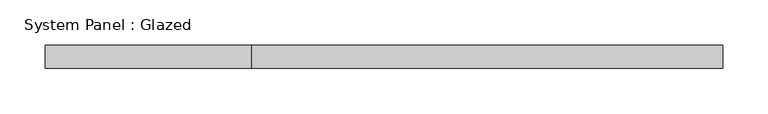
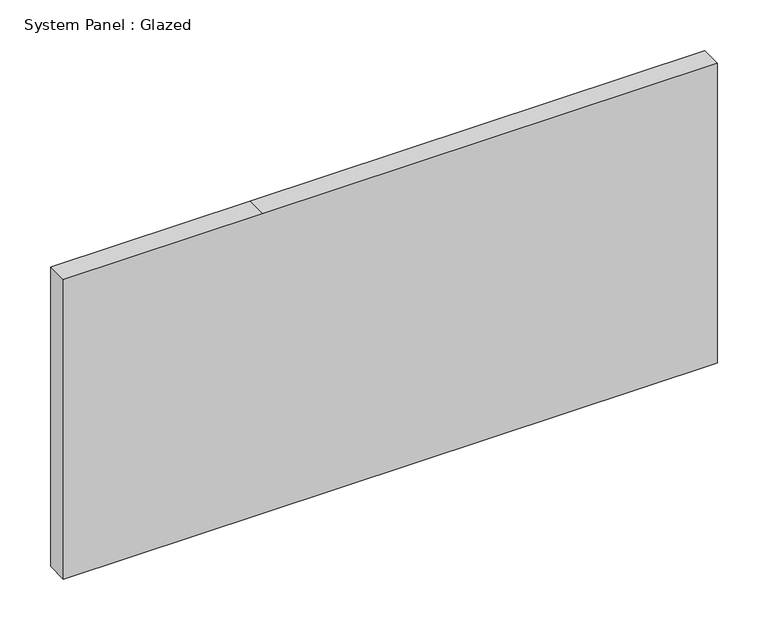
"""IFC4 building model written with IfcOpenShell, lengths in millimetres: plate geometry, System Panel : Glazed."""

from ifc_helpers import new_model, si_unit, frame, origin, place, context, project, spatial, polyline, outline, extrude, source, transform, mapped, element, save


def system_panel_glazed_a3b4e73b(model_context):
    return source(origin(), model_context, "Body", "SweptSolid", [
        extrude(outline(polyline([(0.0, -373.5323778), (0.0, -145.6774593), (0.0, 373.5323778), (361.95, 373.5323778), (361.95, -145.6774593), (361.95, -373.5323778), (0.0, -373.5323778)])), frame((0.0, 19.05, 0.0), z_axis=(0.0, 1.0, 0.0), x_axis=(0.0, 0.0, 1.0)), (0.0, 0.0, 1.0), 25.4),
    ])


if __name__ == "__main__":
    model = new_model("IFC4")
    model_context = context("Model", 3, world=origin())
    ifc_project = project(units=[si_unit("LENGTHUNIT", "METRE", prefix="MILLI")], contexts=[model_context])
    site = spatial("IfcSite", under=ifc_project)
    building = spatial("IfcBuilding", under=site)
    placement = place(None, origin())
    system_panel_glazed_shape = system_panel_glazed_a3b4e73b(model_context)
    element("IfcPlate", 1, ObjectType="System Panel : Glazed", at=placement, inside=building, context=model_context, shape_type="MappedRepresentation", body=[
        mapped(system_panel_glazed_shape, transform((0.0, 0.0, 0.0), x_axis=(1.0, 0.0, 0.0), y_axis=(0.0, 1.0, 0.0), z_axis=(0.0, 0.0, 1.0))),
    ])
    save(model, "model.ifc")

# Revit data of these elements
# Type "System Panel : Glazed"
#   Construction Type Id = "GSP4R"
#   Analytic Construction = "1/8 in Pilkington single glazing"
#   Visual Light Transmittance = 0.9
#   Solar Heat Gain Coefficient = 0.86
#   Heat Transfer Coefficient (U) = 1.18115 BTU/(h·ft²·°F)
#   Define Thermal Properties by = 1
# Element 1 (IfcPlate, "System Panel : Glazed")
#   Materials on its faces: "Glass"
# Materials
#   "Glass": class "Glass", colour RGB 0 128 192, transparency 0.75, Description = "Soda Lime Glass", Cost = 0
